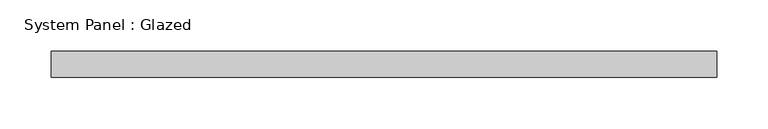
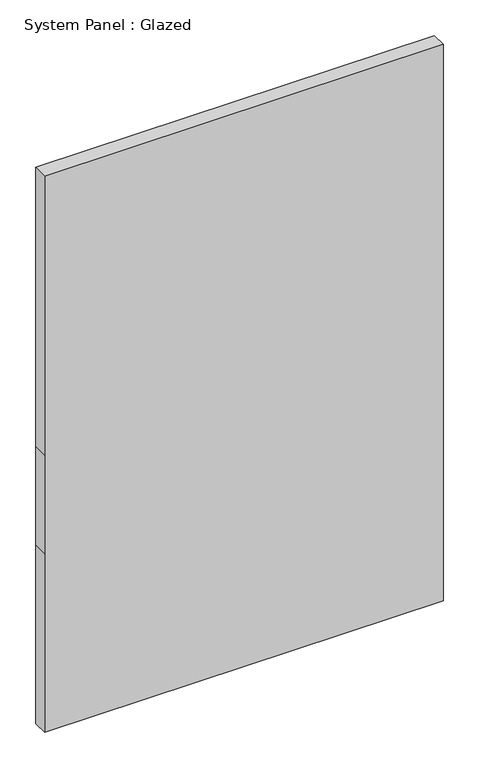
"""IFC4 building model written with IfcOpenShell, lengths in millimetres: plate geometry, System Panel : Glazed."""

from ifc_helpers import new_model, si_unit, frame, origin, place, context, project, spatial, polyline, outline, extrude, source, transform, mapped, element, save


def system_panel_glazed_3bdca378(model_context):
    return source(origin(), model_context, "Body", "SweptSolid", [
        extrude(outline(polyline([(0.0, -323.85), (0.0, 323.85), (307.2248327, 323.85), (476.7122491, 323.85), (955.3870819, 323.85), (955.3870819, -323.85), (476.7122491, -323.85), (307.2248327, -323.85), (0.0, -323.85)])), frame((0.0, 19.05, 0.0), z_axis=(0.0, 1.0, 0.0), x_axis=(0.0, 0.0, 1.0)), (0.0, 0.0, 1.0), 25.4),
    ])


if __name__ == "__main__":
    model = new_model("IFC4")
    model_context = context("Model", 3, world=origin())
    ifc_project = project(units=[si_unit("LENGTHUNIT", "METRE", prefix="MILLI")], contexts=[model_context])
    site = spatial("IfcSite", under=ifc_project)
    building = spatial("IfcBuilding", under=site)
    placement = place(None, origin())
    system_panel_glazed_shape = system_panel_glazed_3bdca378(model_context)
    element("IfcPlate", 1, ObjectType="System Panel : Glazed", at=placement, inside=building, context=model_context, shape_type="MappedRepresentation", body=[
        mapped(system_panel_glazed_shape, transform((0.0, 0.0, 0.0), x_axis=(1.0, 0.0, 0.0), y_axis=(0.0, 1.0, 0.0), z_axis=(0.0, 0.0, 1.0))),
    ])
    save(model, "model.ifc")

# Revit data of these elements
# Type "System Panel : Glazed"
#   Construction Type Id = "GSP4R"
#   Analytic Construction = "1/8 in Pilkington single glazing"
#   Visual Light Transmittance = 0.9
#   Solar Heat Gain Coefficient = 0.86
#   Heat Transfer Coefficient (U) = 1.18115 BTU/(h·ft²·°F)
#   Define Thermal Properties by = 1
# Element 1 (IfcPlate, "System Panel : Glazed")
#   Materials on its faces: "Glass"
# Materials
#   "Glass": class "Glass", colour RGB 0 128 192, transparency 0.75, Description = "Soda Lime Glass", Cost = 0
